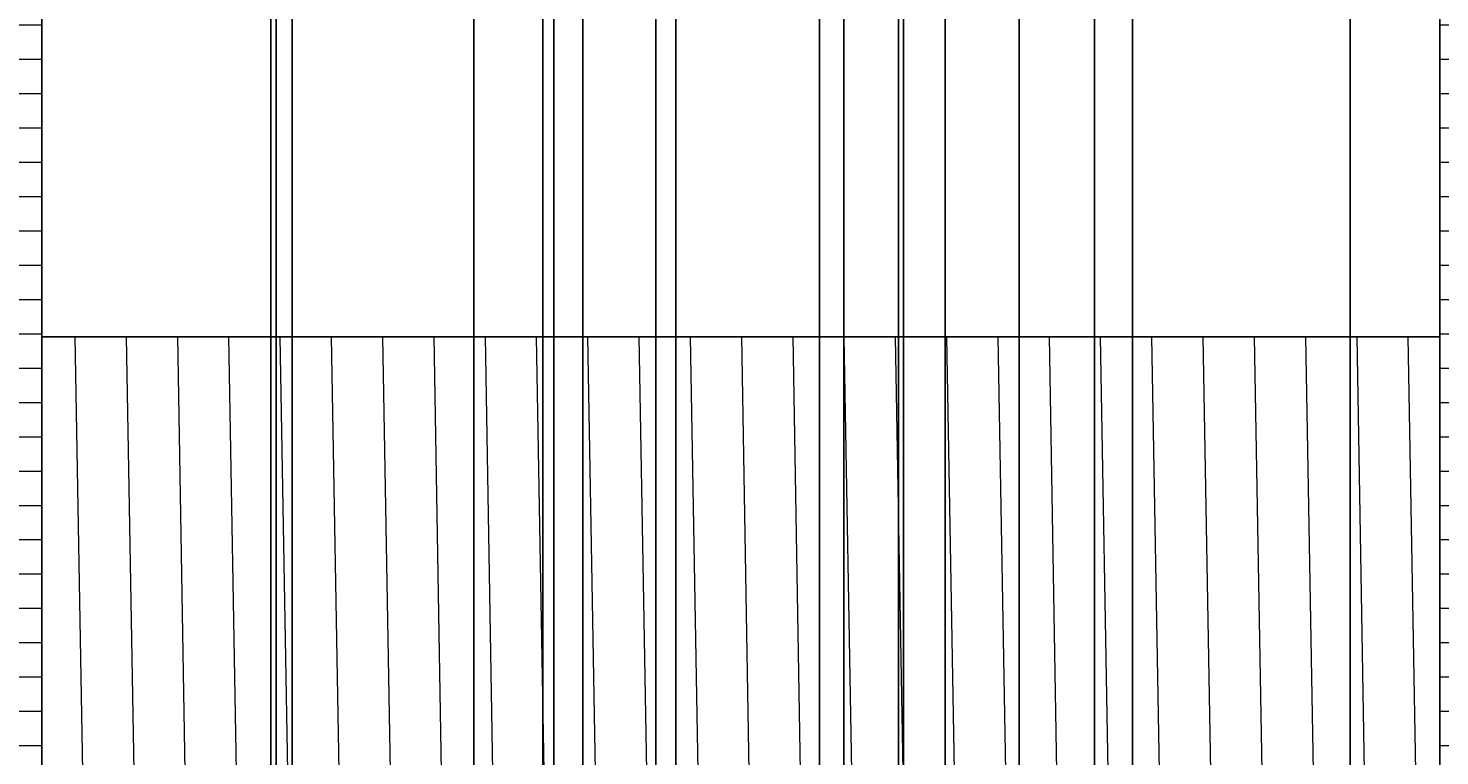
# Model space of a CAD drawing. Units: inches. Extents: x 241 to 943, y 109 to 1396.
# Tile 31 of 34: x 532 to 725, y 1180 to 1279. Entities that reach past the tile are written whole.
import ezdxf

# ---------------------------------------------------------------- set-up
doc = ezdxf.new("R2010")
doc.units = ezdxf.units.IN
doc.header["$MEASUREMENT"] = 0
for name, color, linetype, lineweight in [('A-ANNO-DIMS', 2, 'Continuous', 18), ('A-ELEV', 7, 'Continuous', 25), ('A-GLAZ', 4, 'Continuous', 18), ('A-WALL-PATT', 8, 'Continuous', 13)]:
    doc.layers.add(name, color=color, linetype=linetype, lineweight=lineweight)
doc.styles.get("Standard").update_dxf_attribs({"font": 'arial.ttf'})
doc.dimstyles.get("Standard").update_dxf_attribs({"dimtxt": 1.4375, "dimasz": 0.18, "dimexe": 0.18, "dimexo": 0.0625, "dimgap": 0.09, "dimtad": 0, "dimtih": 1, "dimtoh": 1, "dimdec": 4, "dimzin": 0, "dimdsep": 46, "dimlunit": 4, "dimtxsty": 'Standard', "dimcen": 0.09, "dimadec": 0, "dimazin": 0, "dimtfac": 1, "dimtdec": 4, "dimtofl": 0, "dimtmove": 0, "dimatfit": 3, "dimfxl": 1, "dimtolj": 1, "dimtzin": 0, "dimarcsym": 0})

# ---------------------------------------------------------------- blocks, each defined once
blk = doc.blocks.new('*D12')
at = {"layer": 'A-ANNO-DIMS', "color": 0, "lineweight": -2, "transparency": 16777216}
for p, q in [((530.23, 384.24), (530.23, 1395.05)), ((530.41, 1394.87), (587.56, 1394.87)), ((650.73, 1394.87), (593.58, 1394.87)), ((650.91, 384.24), (650.91, 1395.05))]:
    blk.add_line(p, q, dxfattribs=at)
at = {"layer": 'A-ANNO-DIMS', "color": 0, "transparency": 16777216}
for points in [[(530.41, 1394.9), (530.41, 1394.84), (530.23, 1394.87)], [(650.73, 1394.9), (650.73, 1394.84), (650.91, 1394.87)]]:
    blk.add_solid(points, dxfattribs=at)
at = {"layer": 'Defpoints', "color": 0, "transparency": 16777216}
for p in [(650.91, 1394.87), (530.23, 384.18), (650.91, 384.18)]:
    blk.add_point(p, dxfattribs=at)
at = {"layer": 'A-ANNO-DIMS', "color": 0, "transparency": 16777216, "insert": (590.57, 1394.87), "char_height": 1.438, "attachment_point": 5}
blk.add_mtext('\\A1;120.68', dxfattribs=at)
blk = doc.blocks.new('*D13')
at = {"layer": 'A-ANNO-DIMS', "color": 0, "lineweight": -2, "transparency": 16777216}
for p, q in [((650.91, 384.24), (650.91, 1395.05)), ((651.09, 1394.87), (656.14, 1394.87)), ((667.21, 1394.87), (662.16, 1394.87)), ((667.39, 290.06), (667.39, 1395.05))]:
    blk.add_line(p, q, dxfattribs=at)
at = {"layer": 'A-ANNO-DIMS', "color": 0, "transparency": 16777216}
for points in [[(651.09, 1394.9), (651.09, 1394.84), (650.91, 1394.87)], [(667.21, 1394.9), (667.21, 1394.84), (667.39, 1394.87)]]:
    blk.add_solid(points, dxfattribs=at)
at = {"layer": 'Defpoints', "color": 0, "transparency": 16777216}
for p in [(667.39, 1394.87), (650.91, 384.18), (667.39, 290)]:
    blk.add_point(p, dxfattribs=at)
at = {"layer": 'A-ANNO-DIMS', "color": 0, "transparency": 16777216, "insert": (659.15, 1394.87), "char_height": 1.438, "attachment_point": 5}
blk.add_mtext('\\A1;16.486', dxfattribs=at)
blk = doc.blocks.new('*D14')
at = {"layer": 'A-ANNO-DIMS', "color": 0, "lineweight": -2, "transparency": 16777216}
for p, q in [((667.39, 290.06), (667.39, 1395.05)), ((667.57, 1394.87), (727.7, 1394.87)), ((793.85, 1394.87), (733.72, 1394.87)), ((794.03, 290.06), (794.03, 1395.05))]:
    blk.add_line(p, q, dxfattribs=at)
at = {"layer": 'A-ANNO-DIMS', "color": 0, "transparency": 16777216}
for points in [[(667.57, 1394.9), (667.57, 1394.84), (667.39, 1394.87)], [(793.85, 1394.9), (793.85, 1394.84), (794.03, 1394.87)]]:
    blk.add_solid(points, dxfattribs=at)
at = {"layer": 'Defpoints', "color": 0, "transparency": 16777216}
for p in [(794.03, 1394.87), (667.39, 290), (794.03, 290)]:
    blk.add_point(p, dxfattribs=at)
at = {"layer": 'A-ANNO-DIMS', "color": 0, "transparency": 16777216, "insert": (730.71, 1394.87), "char_height": 1.438, "attachment_point": 5}
blk.add_mtext('\\A1;126.63', dxfattribs=at)
blk = doc.blocks.new('*D57')
at = {"layer": 'A-ANNO-DIMS', "color": 0, "lineweight": -2, "transparency": 16777216}
for p, q in [((508.31, 1070.92), (508.31, 1395.05)), ((508.49, 1394.87), (518.04, 1394.87)), ((533.77, 1394.87), (524.21, 1394.87)), ((533.95, 1108.23), (533.95, 1395.05))]:
    blk.add_line(p, q, dxfattribs=at)
at = {"layer": 'A-ANNO-DIMS', "color": 0, "transparency": 16777216}
for points in [[(508.49, 1394.9), (508.49, 1394.84), (508.31, 1394.87)], [(533.77, 1394.9), (533.77, 1394.84), (533.95, 1394.87)]]:
    blk.add_solid(points, dxfattribs=at)
at = {"layer": 'Defpoints', "color": 0, "transparency": 16777216}
for p in [(533.95, 1394.87), (533.95, 1108.17), (508.31, 1070.85)]:
    blk.add_point(p, dxfattribs=at)
at = {"layer": 'A-ANNO-DIMS', "color": 0, "transparency": 16777216, "insert": (521.13, 1394.87), "char_height": 1.438, "attachment_point": 5}
blk.add_mtext('\\A1;25.646', dxfattribs=at)
blk = doc.blocks.new('*D62')
at = {"layer": 'A-ANNO-DIMS', "color": 0, "lineweight": -2, "transparency": 16777216}
for p, q in [((424.11, 568.89), (424.11, 1395.05)), ((424.29, 1394.87), (492.35, 1394.87)), ((565.02, 1394.87), (496.96, 1394.87)), ((565.2, 568.89), (565.2, 1395.05))]:
    blk.add_line(p, q, dxfattribs=at)
at = {"layer": 'A-ANNO-DIMS', "color": 0, "transparency": 16777216}
for points in [[(424.29, 1394.9), (424.29, 1394.84), (424.11, 1394.87)], [(565.02, 1394.9), (565.02, 1394.84), (565.2, 1394.87)]]:
    blk.add_solid(points, dxfattribs=at)
at = {"layer": 'Defpoints', "color": 0, "transparency": 16777216}
for p in [(565.2, 1394.87), (424.11, 568.83), (565.2, 568.83)]:
    blk.add_point(p, dxfattribs=at)
at = {"layer": 'A-ANNO-DIMS', "color": 0, "transparency": 16777216, "insert": (494.66, 1394.87), "char_height": 1.438, "attachment_point": 5}
blk.add_mtext('\\A1;141.1', dxfattribs=at)
blk = doc.blocks.new('*D63')
at = {"layer": 'A-ANNO-DIMS', "color": 0, "lineweight": -2, "transparency": 16777216}
for p, q in [((651.6, 568.89), (651.6, 1395.05)), ((651.78, 1394.87), (719.84, 1394.87)), ((792.51, 1394.87), (724.45, 1394.87)), ((792.69, 568.89), (792.69, 1395.05))]:
    blk.add_line(p, q, dxfattribs=at)
at = {"layer": 'A-ANNO-DIMS', "color": 0, "transparency": 16777216}
for points in [[(651.78, 1394.9), (651.78, 1394.84), (651.6, 1394.87)], [(792.51, 1394.9), (792.51, 1394.84), (792.69, 1394.87)]]:
    blk.add_solid(points, dxfattribs=at)
at = {"layer": 'Defpoints', "color": 0, "transparency": 16777216}
for p in [(792.69, 1394.87), (651.6, 568.83), (792.69, 568.83)]:
    blk.add_point(p, dxfattribs=at)
at = {"layer": 'A-ANNO-DIMS', "color": 0, "transparency": 16777216, "insert": (722.14, 1394.87), "char_height": 1.438, "attachment_point": 5}
blk.add_mtext('\\A1;141.1', dxfattribs=at)
blk = doc.blocks.new('*D65')
at = {"layer": 'A-ANNO-DIMS', "color": 0, "lineweight": -2, "transparency": 16777216}
for p, q in [((424.11, 700.85), (424.11, 1395.05)), ((424.29, 1394.87), (505.52, 1394.87)), ((592.77, 1394.87), (511.54, 1394.87)), ((592.95, 700.85), (592.95, 1395.05))]:
    blk.add_line(p, q, dxfattribs=at)
at = {"layer": 'A-ANNO-DIMS', "color": 0, "transparency": 16777216}
for points in [[(424.29, 1394.9), (424.29, 1394.84), (424.11, 1394.87)], [(592.77, 1394.9), (592.77, 1394.84), (592.95, 1394.87)]]:
    blk.add_solid(points, dxfattribs=at)
at = {"layer": 'Defpoints', "color": 0, "transparency": 16777216}
for p in [(592.95, 1394.87), (424.11, 700.79), (592.95, 700.79)]:
    blk.add_point(p, dxfattribs=at)
at = {"layer": 'A-ANNO-DIMS', "color": 0, "transparency": 16777216, "insert": (508.53, 1394.87), "char_height": 1.438, "attachment_point": 5}
blk.add_mtext('\\A1;168.85', dxfattribs=at)
blk = doc.blocks.new('*D66')
at = {"layer": 'A-ANNO-DIMS', "color": 0, "lineweight": -2, "transparency": 16777216}
for p, q in [((617.76, 702.85), (617.76, 1395.05)), ((617.94, 1394.87), (680.69, 1394.87)), ((749.45, 1394.87), (686.7, 1394.87)), ((749.63, 702.85), (749.63, 1395.05))]:
    blk.add_line(p, q, dxfattribs=at)
at = {"layer": 'A-ANNO-DIMS', "color": 0, "transparency": 16777216}
for points in [[(617.94, 1394.9), (617.94, 1394.84), (617.76, 1394.87)], [(749.45, 1394.9), (749.45, 1394.84), (749.63, 1394.87)]]:
    blk.add_solid(points, dxfattribs=at)
at = {"layer": 'Defpoints', "color": 0, "transparency": 16777216}
for p in [(749.63, 1394.87), (617.76, 702.79), (749.63, 702.79)]:
    blk.add_point(p, dxfattribs=at)
at = {"layer": 'A-ANNO-DIMS', "color": 0, "transparency": 16777216, "insert": (683.7, 1394.87), "char_height": 1.438, "attachment_point": 5}
blk.add_mtext('\\A1;131.87', dxfattribs=at)
blk = doc.blocks.new('*D67')
at = {"layer": 'A-ANNO-DIMS', "color": 0, "lineweight": -2, "transparency": 16777216}
for p, q in [((389.04, 773.55), (389.04, 1395.05)), ((389.22, 1394.87), (495.34, 1394.87)), ((607.64, 1394.87), (501.52, 1394.87)), ((607.82, 773.55), (607.82, 1395.05))]:
    blk.add_line(p, q, dxfattribs=at)
at = {"layer": 'A-ANNO-DIMS', "color": 0, "transparency": 16777216}
for points in [[(389.22, 1394.9), (389.22, 1394.84), (389.04, 1394.87)], [(607.64, 1394.9), (607.64, 1394.84), (607.82, 1394.87)]]:
    blk.add_solid(points, dxfattribs=at)
at = {"layer": 'Defpoints', "color": 0, "transparency": 16777216}
for p in [(607.82, 1394.87), (389.04, 773.49), (607.82, 773.49)]:
    blk.add_point(p, dxfattribs=at)
at = {"layer": 'A-ANNO-DIMS', "color": 0, "transparency": 16777216, "insert": (498.43, 1394.87), "char_height": 1.438, "attachment_point": 5}
blk.add_mtext('\\A1;218.77', dxfattribs=at)
blk = doc.blocks.new('*D68')
at = {"layer": 'A-ANNO-DIMS', "color": 0, "lineweight": -2, "transparency": 16777216}
for p, q in [((617.76, 841.6), (617.76, 1395.05)), ((617.94, 1394.87), (702.22, 1394.87)), ((792.51, 1394.87), (708.23, 1394.87)), ((792.69, 841.6), (792.69, 1395.05))]:
    blk.add_line(p, q, dxfattribs=at)
at = {"layer": 'A-ANNO-DIMS', "color": 0, "transparency": 16777216}
for points in [[(617.94, 1394.9), (617.94, 1394.84), (617.76, 1394.87)], [(792.51, 1394.9), (792.51, 1394.84), (792.69, 1394.87)]]:
    blk.add_solid(points, dxfattribs=at)
at = {"layer": 'Defpoints', "color": 0, "transparency": 16777216}
for p in [(792.69, 1394.87), (617.76, 841.54), (792.69, 841.54)]:
    blk.add_point(p, dxfattribs=at)
at = {"layer": 'A-ANNO-DIMS', "color": 0, "transparency": 16777216, "insert": (705.23, 1394.87), "char_height": 1.438, "attachment_point": 5}
blk.add_mtext('\\A1;174.93', dxfattribs=at)
blk = doc.blocks.new('*D69')
at = {"layer": 'A-ANNO-DIMS', "color": 0, "lineweight": -2, "transparency": 16777216}
for p, q in [((389.04, 941.55), (389.04, 1395.05)), ((389.22, 1394.87), (476.28, 1394.87)), ((567.95, 1394.87), (480.9, 1394.87)), ((568.13, 941.55), (568.13, 1395.05))]:
    blk.add_line(p, q, dxfattribs=at)
at = {"layer": 'A-ANNO-DIMS', "color": 0, "transparency": 16777216}
for points in [[(389.22, 1394.9), (389.22, 1394.84), (389.04, 1394.87)], [(567.95, 1394.9), (567.95, 1394.84), (568.13, 1394.87)]]:
    blk.add_solid(points, dxfattribs=at)
at = {"layer": 'Defpoints', "color": 0, "transparency": 16777216}
for p in [(568.13, 1394.87), (389.04, 941.49), (568.13, 941.49)]:
    blk.add_point(p, dxfattribs=at)
at = {"layer": 'A-ANNO-DIMS', "color": 0, "transparency": 16777216, "insert": (478.59, 1394.87), "char_height": 1.438, "attachment_point": 5}
blk.add_mtext('\\A1;179.1', dxfattribs=at)
blk = doc.blocks.new('*D70')
at = {"layer": 'A-ANNO-DIMS', "color": 0, "lineweight": -2, "transparency": 16777216}
for p, q in [((603.87, 1009.6), (603.87, 1395.05)), ((604.05, 1394.87), (674.69, 1394.87)), ((751.33, 1394.87), (680.69, 1394.87)), ((751.51, 1009.6), (751.51, 1395.05))]:
    blk.add_line(p, q, dxfattribs=at)
at = {"layer": 'A-ANNO-DIMS', "color": 0, "transparency": 16777216}
for points in [[(604.05, 1394.9), (604.05, 1394.84), (603.87, 1394.87)], [(751.33, 1394.9), (751.33, 1394.84), (751.51, 1394.87)]]:
    blk.add_solid(points, dxfattribs=at)
at = {"layer": 'Defpoints', "color": 0, "transparency": 16777216}
for p in [(751.51, 1394.87), (603.87, 1009.54), (751.51, 1009.54)]:
    blk.add_point(p, dxfattribs=at)
at = {"layer": 'A-ANNO-DIMS', "color": 0, "transparency": 16777216, "insert": (677.69, 1394.87), "char_height": 1.438, "attachment_point": 5}
blk.add_mtext('\\A1;147.64', dxfattribs=at)
blk = doc.blocks.new('*D82')
at = {"layer": 'A-ANNO-DIMS', "color": 0, "lineweight": -2, "transparency": 16777216}
for p, q in [((565.2, 568.89), (565.2, 1395.05)), ((565.38, 1394.87), (605.89, 1394.87)), ((651.42, 1394.87), (610.91, 1394.87)), ((651.6, 568.89), (651.6, 1395.05))]:
    blk.add_line(p, q, dxfattribs=at)
at = {"layer": 'A-ANNO-DIMS', "color": 0, "transparency": 16777216}
for points in [[(565.38, 1394.9), (565.38, 1394.84), (565.2, 1394.87)], [(651.42, 1394.9), (651.42, 1394.84), (651.6, 1394.87)]]:
    blk.add_solid(points, dxfattribs=at)
at = {"layer": 'Defpoints', "color": 0, "transparency": 16777216}
for p in [(651.6, 1394.87), (565.2, 568.83), (651.6, 568.83)]:
    blk.add_point(p, dxfattribs=at)
at = {"layer": 'A-ANNO-DIMS', "color": 0, "transparency": 16777216, "insert": (608.4, 1394.87), "char_height": 1.438, "attachment_point": 5}
blk.add_mtext('\\A1;86.40', dxfattribs=at)
blk = doc.blocks.new('*D83')
at = {"layer": 'A-ANNO-DIMS', "color": 0, "lineweight": -2, "transparency": 16777216}
for p, q in [((592.95, 700.85), (592.95, 1395.05)), ((593.13, 1394.87), (602.27, 1394.87)), ((617.58, 1394.87), (608.45, 1394.87)), ((617.76, 702.85), (617.76, 1395.05))]:
    blk.add_line(p, q, dxfattribs=at)
at = {"layer": 'A-ANNO-DIMS', "color": 0, "transparency": 16777216}
for points in [[(593.13, 1394.9), (593.13, 1394.84), (592.95, 1394.87)], [(617.58, 1394.9), (617.58, 1394.84), (617.76, 1394.87)]]:
    blk.add_solid(points, dxfattribs=at)
at = {"layer": 'Defpoints', "color": 0, "transparency": 16777216}
for p in [(617.76, 1394.87), (617.76, 702.79), (592.95, 700.79)]:
    blk.add_point(p, dxfattribs=at)
at = {"layer": 'A-ANNO-DIMS', "color": 0, "transparency": 16777216, "insert": (605.36, 1394.87), "char_height": 1.438, "attachment_point": 5}
blk.add_mtext('\\A1;24.805', dxfattribs=at)
blk = doc.blocks.new('*D89')
at = {"layer": 'A-ANNO-DIMS', "color": 0, "lineweight": -2, "transparency": 16777216}
for p, q in [((377.04, 841.6), (377.04, 1395.05)), ((377.22, 1394.87), (494.32, 1394.87)), ((617.58, 1394.87), (500.48, 1394.87)), ((617.76, 841.6), (617.76, 1395.05))]:
    blk.add_line(p, q, dxfattribs=at)
at = {"layer": 'A-ANNO-DIMS', "color": 0, "transparency": 16777216}
for points in [[(377.22, 1394.9), (377.22, 1394.84), (377.04, 1394.87)], [(617.58, 1394.9), (617.58, 1394.84), (617.76, 1394.87)]]:
    blk.add_solid(points, dxfattribs=at)
at = {"layer": 'Defpoints', "color": 0, "transparency": 16777216}
for p in [(617.76, 1394.87), (377.04, 841.54), (617.76, 841.54)]:
    blk.add_point(p, dxfattribs=at)
at = {"layer": 'A-ANNO-DIMS', "color": 0, "transparency": 16777216, "insert": (497.4, 1394.87), "char_height": 1.438, "attachment_point": 5}
blk.add_mtext('\\A1;240.72', dxfattribs=at)
blk = doc.blocks.new('*D90')
at = {"layer": 'A-ANNO-DIMS', "color": 0, "lineweight": -2, "transparency": 16777216}
for p, q in [((568.13, 941.55), (568.13, 1395.05)), ((568.31, 1394.87), (582.92, 1394.87)), ((603.69, 1394.87), (589.08, 1394.87)), ((603.87, 902.92), (603.87, 1395.05))]:
    blk.add_line(p, q, dxfattribs=at)
at = {"layer": 'A-ANNO-DIMS', "color": 0, "transparency": 16777216}
for points in [[(568.31, 1394.9), (568.31, 1394.84), (568.13, 1394.87)], [(603.69, 1394.9), (603.69, 1394.84), (603.87, 1394.87)]]:
    blk.add_solid(points, dxfattribs=at)
at = {"layer": 'Defpoints', "color": 0, "transparency": 16777216}
for p in [(603.87, 1394.87), (568.13, 941.49), (603.87, 902.85)]:
    blk.add_point(p, dxfattribs=at)
at = {"layer": 'A-ANNO-DIMS', "color": 0, "transparency": 16777216, "insert": (586, 1394.87), "char_height": 1.438, "attachment_point": 5}
blk.add_mtext('\\A1;35.735', dxfattribs=at)
blk = doc.blocks.new('*D99')
at = {"layer": 'A-ANNO-DIMS', "color": 0, "lineweight": -2, "transparency": 16777216}
for p, q in [((417.09, 181.71), (417.09, 1395.05)), ((417.27, 1394.87), (539.16, 1394.87)), ((667.21, 1394.87), (545.33, 1394.87)), ((667.39, 214.58), (667.39, 1395.05))]:
    blk.add_line(p, q, dxfattribs=at)
at = {"layer": 'A-ANNO-DIMS', "color": 0, "transparency": 16777216}
for points in [[(417.27, 1394.9), (417.27, 1394.84), (417.09, 1394.87)], [(667.21, 1394.9), (667.21, 1394.84), (667.39, 1394.87)]]:
    blk.add_solid(points, dxfattribs=at)
at = {"layer": 'Defpoints', "color": 0, "transparency": 16777216}
for p in [(667.39, 1394.87), (667.39, 214.52), (417.09, 181.65)]:
    blk.add_point(p, dxfattribs=at)
at = {"layer": 'A-ANNO-DIMS', "color": 0, "transparency": 16777216, "insert": (542.24, 1394.87), "char_height": 1.438, "attachment_point": 5}
blk.add_mtext('\\A1;250.30', dxfattribs=at)
blk = doc.blocks.new('*D104')
at = {"layer": 'A-ANNO-DIMS', "color": 0, "lineweight": -2, "transparency": 16777216}
for p, q in [((533.95, 1108.23), (533.95, 1395.05)), ((534.13, 1394.87), (546.87, 1394.87)), ((565.77, 1394.87), (553.03, 1394.87)), ((565.95, 1110.23), (565.95, 1395.05))]:
    blk.add_line(p, q, dxfattribs=at)
at = {"layer": 'A-ANNO-DIMS', "color": 0, "transparency": 16777216}
for points in [[(534.13, 1394.9), (534.13, 1394.84), (533.95, 1394.87)], [(565.77, 1394.9), (565.77, 1394.84), (565.95, 1394.87)]]:
    blk.add_solid(points, dxfattribs=at)
at = {"layer": 'Defpoints', "color": 0, "transparency": 16777216}
for p in [(565.95, 1394.87), (565.95, 1110.17), (533.95, 1108.17)]:
    blk.add_point(p, dxfattribs=at)
at = {"layer": 'A-ANNO-DIMS', "color": 0, "transparency": 16777216, "insert": (549.95, 1394.87), "char_height": 1.438, "attachment_point": 5}
blk.add_mtext('\\A1;31.995', dxfattribs=at)
blk = doc.blocks.new('*D105')
at = {"layer": 'A-ANNO-DIMS', "color": 0, "lineweight": -2, "transparency": 16777216}
for p, q in [((565.95, 1110.23), (565.95, 1395.05)), ((566.13, 1394.87), (581.08, 1394.87)), ((602.18, 1394.87), (587.23, 1394.87)), ((602.36, 1110.23), (602.36, 1395.05))]:
    blk.add_line(p, q, dxfattribs=at)
at = {"layer": 'A-ANNO-DIMS', "color": 0, "transparency": 16777216}
for points in [[(566.13, 1394.9), (566.13, 1394.84), (565.95, 1394.87)], [(602.18, 1394.9), (602.18, 1394.84), (602.36, 1394.87)]]:
    blk.add_solid(points, dxfattribs=at)
at = {"layer": 'Defpoints', "color": 0, "transparency": 16777216}
for p in [(602.36, 1394.87), (565.95, 1110.17), (602.36, 1110.17)]:
    blk.add_point(p, dxfattribs=at)
at = {"layer": 'A-ANNO-DIMS', "color": 0, "transparency": 16777216, "insert": (584.15, 1394.87), "char_height": 1.438, "attachment_point": 5}
blk.add_mtext('\\A1;36.415', dxfattribs=at)
blk = doc.blocks.new('*D106')
at = {"layer": 'A-ANNO-DIMS', "color": 0, "lineweight": -2, "transparency": 16777216}
for p, q in [((602.36, 1110.23), (602.36, 1395.05)), ((602.54, 1394.87), (608.99, 1394.87)), ((620.34, 1394.87), (613.89, 1394.87)), ((620.52, 1110.23), (620.52, 1395.05))]:
    blk.add_line(p, q, dxfattribs=at)
at = {"layer": 'A-ANNO-DIMS', "color": 0, "transparency": 16777216}
for points in [[(602.54, 1394.9), (602.54, 1394.84), (602.36, 1394.87)], [(620.34, 1394.9), (620.34, 1394.84), (620.52, 1394.87)]]:
    blk.add_solid(points, dxfattribs=at)
at = {"layer": 'Defpoints', "color": 0, "transparency": 16777216}
for p in [(620.52, 1394.87), (602.36, 1110.17), (620.52, 1110.17)]:
    blk.add_point(p, dxfattribs=at)
at = {"layer": 'A-ANNO-DIMS', "color": 0, "transparency": 16777216, "insert": (611.44, 1394.87), "char_height": 1.438, "attachment_point": 5}
blk.add_mtext('\\A1;18.16', dxfattribs=at)
blk = doc.blocks.new('*D107')
at = {"layer": 'A-ANNO-DIMS', "color": 0, "lineweight": -2, "transparency": 16777216}
for p, q in [((620.52, 1110.23), (620.52, 1395.05)), ((620.7, 1394.87), (628.91, 1394.87)), ((643.27, 1394.87), (635.07, 1394.87)), ((643.45, 1110.23), (643.45, 1395.05))]:
    blk.add_line(p, q, dxfattribs=at)
at = {"layer": 'A-ANNO-DIMS', "color": 0, "transparency": 16777216}
for points in [[(620.7, 1394.9), (620.7, 1394.84), (620.52, 1394.87)], [(643.27, 1394.9), (643.27, 1394.84), (643.45, 1394.87)]]:
    blk.add_solid(points, dxfattribs=at)
at = {"layer": 'Defpoints', "color": 0, "transparency": 16777216}
for p in [(643.45, 1394.87), (620.52, 1110.17), (643.45, 1110.17)]:
    blk.add_point(p, dxfattribs=at)
at = {"layer": 'A-ANNO-DIMS', "color": 0, "transparency": 16777216, "insert": (631.99, 1394.87), "char_height": 1.438, "attachment_point": 5}
blk.add_mtext('\\A1;22.932', dxfattribs=at)
blk = doc.blocks.new('*D108')
at = {"layer": 'A-ANNO-DIMS', "color": 0, "lineweight": -2, "transparency": 16777216}
for p, q in [((643.45, 1110.23), (643.45, 1395.05)), ((643.63, 1394.87), (660.66, 1394.87)), ((682.69, 1394.87), (665.67, 1394.87)), ((682.87, 1110.23), (682.87, 1395.05))]:
    blk.add_line(p, q, dxfattribs=at)
at = {"layer": 'A-ANNO-DIMS', "color": 0, "transparency": 16777216}
for points in [[(643.63, 1394.9), (643.63, 1394.84), (643.45, 1394.87)], [(682.69, 1394.9), (682.69, 1394.84), (682.87, 1394.87)]]:
    blk.add_solid(points, dxfattribs=at)
at = {"layer": 'Defpoints', "color": 0, "transparency": 16777216}
for p in [(682.87, 1394.87), (643.45, 1110.17), (682.87, 1110.17)]:
    blk.add_point(p, dxfattribs=at)
at = {"layer": 'A-ANNO-DIMS', "color": 0, "transparency": 16777216, "insert": (663.16, 1394.87), "char_height": 1.438, "attachment_point": 5}
blk.add_mtext('\\A1;39.42', dxfattribs=at)
blk = doc.blocks.new('*D109')
at = {"layer": 'A-ANNO-DIMS', "color": 0, "lineweight": -2, "transparency": 16777216}
for p, q in [((682.87, 1110.23), (682.87, 1395.05)), ((683.05, 1394.87), (701.31, 1394.87)), ((724.64, 1394.87), (706.39, 1394.87)), ((724.82, 1108.23), (724.82, 1395.05))]:
    blk.add_line(p, q, dxfattribs=at)
at = {"layer": 'A-ANNO-DIMS', "color": 0, "transparency": 16777216}
for points in [[(683.05, 1394.9), (683.05, 1394.84), (682.87, 1394.87)], [(724.64, 1394.9), (724.64, 1394.84), (724.82, 1394.87)]]:
    blk.add_solid(points, dxfattribs=at)
at = {"layer": 'Defpoints', "color": 0, "transparency": 16777216}
for p in [(724.82, 1394.87), (682.87, 1110.17), (724.82, 1108.17)]:
    blk.add_point(p, dxfattribs=at)
at = {"layer": 'A-ANNO-DIMS', "color": 0, "transparency": 16777216, "insert": (703.85, 1394.87), "char_height": 1.438, "attachment_point": 5}
blk.add_mtext('\\A1;41.94', dxfattribs=at)
blk = doc.blocks.new('*D113')
at = {"layer": 'A-ANNO-DIMS', "color": 0, "lineweight": -2, "transparency": 16777216}
for p, q in [((603.87, 902.92), (603.87, 1395.05)), ((604.05, 1394.87), (618.91, 1394.87)), ((639.93, 1394.87), (625.07, 1394.87)), ((640.11, 902.92), (640.11, 1395.05))]:
    blk.add_line(p, q, dxfattribs=at)
at = {"layer": 'A-ANNO-DIMS', "color": 0, "transparency": 16777216}
for points in [[(604.05, 1394.9), (604.05, 1394.84), (603.87, 1394.87)], [(639.93, 1394.9), (639.93, 1394.84), (640.11, 1394.87)]]:
    blk.add_solid(points, dxfattribs=at)
at = {"layer": 'Defpoints', "color": 0, "transparency": 16777216}
for p in [(640.11, 1394.87), (603.87, 902.85), (640.11, 902.85)]:
    blk.add_point(p, dxfattribs=at)
at = {"layer": 'A-ANNO-DIMS', "color": 0, "transparency": 16777216, "insert": (621.99, 1394.87), "char_height": 1.438, "attachment_point": 5}
blk.add_mtext('\\A1;36.245', dxfattribs=at)
blk = doc.blocks.new('*D114')
at = {"layer": 'A-ANNO-DIMS', "color": 0, "lineweight": -2, "transparency": 16777216}
for p, q in [((640.11, 902.92), (640.11, 1395.05)), ((640.29, 1394.87), (646.25, 1394.87)), ((657.11, 1394.87), (651.15, 1394.87)), ((657.29, 902.92), (657.29, 1395.05))]:
    blk.add_line(p, q, dxfattribs=at)
at = {"layer": 'A-ANNO-DIMS', "color": 0, "transparency": 16777216}
for points in [[(640.29, 1394.9), (640.29, 1394.84), (640.11, 1394.87)], [(657.11, 1394.9), (657.11, 1394.84), (657.29, 1394.87)]]:
    blk.add_solid(points, dxfattribs=at)
at = {"layer": 'Defpoints', "color": 0, "transparency": 16777216}
for p in [(657.29, 1394.87), (640.11, 902.85), (657.29, 902.85)]:
    blk.add_point(p, dxfattribs=at)
at = {"layer": 'A-ANNO-DIMS', "color": 0, "transparency": 16777216, "insert": (648.7, 1394.87), "char_height": 1.438, "attachment_point": 5}
blk.add_mtext('\\A1;17.18', dxfattribs=at)
blk = doc.blocks.new('*D115')
at = {"layer": 'A-ANNO-DIMS', "color": 0, "lineweight": -2, "transparency": 16777216}
for p, q in [((657.29, 902.92), (657.29, 1395.05)), ((657.47, 1394.87), (664.4, 1394.87)), ((677.51, 1394.87), (670.58, 1394.87)), ((677.69, 902.92), (677.69, 1395.05))]:
    blk.add_line(p, q, dxfattribs=at)
at = {"layer": 'A-ANNO-DIMS', "color": 0, "transparency": 16777216}
for points in [[(657.47, 1394.9), (657.47, 1394.84), (657.29, 1394.87)], [(677.51, 1394.9), (677.51, 1394.84), (677.69, 1394.87)]]:
    blk.add_solid(points, dxfattribs=at)
at = {"layer": 'Defpoints', "color": 0, "transparency": 16777216}
for p in [(677.69, 1394.87), (657.29, 902.85), (677.69, 902.85)]:
    blk.add_point(p, dxfattribs=at)
at = {"layer": 'A-ANNO-DIMS', "color": 0, "transparency": 16777216, "insert": (667.49, 1394.87), "char_height": 1.438, "attachment_point": 5}
blk.add_mtext('\\A1;20.396', dxfattribs=at)
blk = doc.blocks.new('*D116')
at = {"layer": 'A-ANNO-DIMS', "color": 0, "lineweight": -2, "transparency": 16777216}
for p, q in [((677.69, 902.92), (677.69, 1395.05)), ((677.87, 1394.87), (692.06, 1394.87)), ((712.4, 1394.87), (698.22, 1394.87)), ((712.58, 902.92), (712.58, 1395.05))]:
    blk.add_line(p, q, dxfattribs=at)
at = {"layer": 'A-ANNO-DIMS', "color": 0, "transparency": 16777216}
for points in [[(677.87, 1394.9), (677.87, 1394.84), (677.69, 1394.87)], [(712.4, 1394.9), (712.4, 1394.84), (712.58, 1394.87)]]:
    blk.add_solid(points, dxfattribs=at)
at = {"layer": 'Defpoints', "color": 0, "transparency": 16777216}
for p in [(712.58, 1394.87), (677.69, 902.85), (712.58, 902.85)]:
    blk.add_point(p, dxfattribs=at)
at = {"layer": 'A-ANNO-DIMS', "color": 0, "transparency": 16777216, "insert": (695.14, 1394.87), "char_height": 1.438, "attachment_point": 5}
blk.add_mtext('\\A1;34.895', dxfattribs=at)
blk = doc.blocks.new('*D117')
at = {"layer": 'A-ANNO-DIMS', "color": 0, "lineweight": -2, "transparency": 16777216}
for p, q in [((712.58, 902.92), (712.58, 1395.05)), ((712.76, 1394.87), (729.54, 1394.87)), ((751.33, 1394.87), (734.55, 1394.87)), ((751.51, 902.92), (751.51, 1395.05))]:
    blk.add_line(p, q, dxfattribs=at)
at = {"layer": 'A-ANNO-DIMS', "color": 0, "transparency": 16777216}
for points in [[(712.76, 1394.9), (712.76, 1394.84), (712.58, 1394.87)], [(751.33, 1394.9), (751.33, 1394.84), (751.51, 1394.87)]]:
    blk.add_solid(points, dxfattribs=at)
at = {"layer": 'Defpoints', "color": 0, "transparency": 16777216}
for p in [(751.51, 1394.87), (712.58, 902.85), (751.51, 902.85)]:
    blk.add_point(p, dxfattribs=at)
at = {"layer": 'A-ANNO-DIMS', "color": 0, "transparency": 16777216, "insert": (732.05, 1394.87), "char_height": 1.438, "attachment_point": 5}
blk.add_mtext('\\A1;38.92', dxfattribs=at)

msp = doc.modelspace()

# ---------------------------------------------------------------- hatches: boundary and pattern name
at = {"layer": 'A-WALL-PATT'}
h = msp.add_hatch(dxfattribs=at)
h.set_pattern_fill('GRATE', color=256, scale=150)
h.paths.add_polyline_path([(747.7579, 1238.8538), (747.7579, 1275.9142), (747.7579, 1336.1154), (508.3064, 1336.1154), (508.3064, 1275.9142), (508.3064, 1238.8538), (508.3064, 1177.5382), (508.3064, 1109.4916), (508.3064, 1070.8538), (553.5166, 1070.8538), (749.6328, 1070.8538)])
h.paths.add_polyline_path([(533.952, 1108.1686), (533.952, 1177.7336), (533.952, 1303.0286), (724.819, 1303.0286), (724.819, 1108.1686)], flags=16)
h.paths.add_polyline_path([(535.952, 1110.1686), (535.952, 1175.7336), (722.819, 1175.7336), (722.819, 1110.1686)], flags=0)
h.paths.add_polyline_path([(643.4534, 1134.0739), (622.521, 1134.0739), (622.521, 1136.0739), (643.4534, 1136.0739)], flags=0)
h.paths.add_polyline_path([(617.7594, 568.8295), (617.7594, 734.8538), (377.0391, 734.8538), (377.0391, 566.8538), (377.0391, 400.8295), (417.0913, 400.8295), (618.9643, 400.8295)])
h.paths.add_polyline_path([(424.1086, 496.4395), (424.1086, 568.8295), (565.2023, 568.8295), (565.2023, 496.4395)], flags=16)
h.paths.add_polyline_path([(426.1086, 498.4395), (426.1086, 566.8295), (563.2023, 566.8295), (563.2023, 508.9074), (563.2023, 498.4395)], flags=0)
h.paths.add_polyline_path([(508.0803, 508.9074), (508.0803, 519.3754), (450.9259, 519.3754), (450.9259, 525.3816), (445.5808, 525.3816, -1), (445.5808, 527.3816), (450.9259, 527.3816), (450.9259, 566.8295), (508.0803, 566.8295), (537.4269, 566.8295), (537.4269, 508.9074)], flags=0)
h.paths.add_polyline_path([(506.0803, 521.3754), (452.9259, 521.3754), (452.9259, 564.8295), (506.0803, 564.8295)], flags=0)
h.paths.add_polyline_path([(424.1086, 628.4013), (424.1086, 700.7912), (592.9542, 700.7912), (592.9542, 628.4013)], flags=16)
h.paths.add_polyline_path([(426.1086, 630.4013), (426.1086, 698.7912), (590.8792, 698.7912), (590.8792, 630.4013)], flags=0)
h.paths.add_polyline_path([(508.1906, 651.3371), (508.0803, 651.3371), (450.9259, 651.3371), (428.0291, 651.3371), (428.0291, 698.7912), (451.9767, 698.7912), (508.0803, 698.7912), (537.4269, 698.7912), (563.2023, 698.7912), (563.2023, 659.3434), (563.9297, 659.3434), (563.9297, 651.3371)], flags=0)
h.paths.add_polyline_path([(506.0803, 653.3371), (452.9259, 653.3371), (452.9259, 657.3434), (445.5808, 657.3434, -1), (445.5808, 659.3434), (452.9259, 659.3434), (452.9259, 696.7912), (506.0803, 696.7912)], flags=0)
h = msp.add_hatch(dxfattribs=at)
h.set_pattern_fill('ANSI31', color=256, scale=56, angle=46)
h.paths.add_polyline_path([(508.3064, 1275.9142), (377.0391, 1275.9142), (377.0391, 1238.8538), (508.3064, 1238.8538)])
h.paths.add_polyline_path([(724.819, 1237.0695), (533.952, 1237.0695), (533.952, 1177.7336), (724.819, 1177.7336)])

# ---------------------------------------------------------------- linework, layer by layer
at = {"layer": 'A-ELEV'}
msp.add_line((533.952, 1237.0695), (724.819, 1237.0695), dxfattribs=at)
at = {"layer": 'A-GLAZ'}
msp.add_lwpolyline([(533.952, 1303.0286), (724.819, 1303.0286), (724.819, 1108.1686), (533.952, 1108.1686)], close=True, dxfattribs=at)

# ---------------------------------------------------------------- dimensions: what is measured, and where the dimension line sits
at = {"layer": 'A-ANNO-DIMS'}
for base, p1, p2, override, picture, middle in [((617.7594, 1394.8654), (377.0391, 841.5382), (617.7594, 841.5382), {"dimdec": 2, "dimlfac": 1, "dimrnd": 0, "dimzin": 0, "dimdsep": 46, "dimlunit": 2}, '*D89', (497.3993, 1394.8654)), ((607.8162, 1394.8654), (389.0429, 773.4916), (607.8162, 773.4916), {"dimdec": 2, "dimlfac": 1, "dimrnd": 0, "dimzin": 0, "dimdsep": 46, "dimlunit": 2}, '*D67', (498.4295, 1394.8654)), ((568.1348, 1394.8654), (389.0429, 941.4916), (568.1348, 941.4916), {"dimdec": 1, "dimlfac": 1, "dimrnd": 0, "dimzin": 0, "dimdsep": 46, "dimlunit": 2}, '*D69', (478.5888, 1394.8654)), ((667.3935, 1394.8654), (417.0913, 181.649), (667.3935, 214.5189), {"dimdec": 2, "dimlfac": 1, "dimrnd": 0, "dimzin": 0, "dimdsep": 46, "dimlunit": 2}, '*D99', (542.2424, 1394.8654)), ((565.2023, 1394.8654), (424.1086, 568.8295), (565.2023, 568.8295), {"dimdec": 1, "dimlfac": 1, "dimrnd": 0, "dimzin": 0, "dimdsep": 46, "dimlunit": 2}, '*D62', (494.6554, 1394.8654)), ((592.9542, 1394.8654), (424.1086, 700.7912), (592.9542, 700.7912), {"dimdec": 2, "dimlfac": 1, "dimrnd": 0, "dimzin": 0, "dimdsep": 46, "dimlunit": 2}, '*D65', (508.5314, 1394.8654)), ((533.952, 1394.8654), (508.3064, 1070.8538), (533.952, 1108.1686), {"dimdec": 3, "dimlfac": 1, "dimrnd": 0, "dimzin": 0, "dimdsep": 46, "dimlunit": 2}, '*D57', (521.1292, 1394.8654)), ((650.907, 1394.8654), (530.2303, 384.1784), (650.907, 384.1784), {"dimdec": 2, "dimlfac": 1, "dimrnd": 0, "dimzin": 0, "dimdsep": 46, "dimlunit": 2}, '*D12', (590.5686, 1394.8654)), ((565.947, 1394.8654), (533.952, 1108.1686), (565.947, 1110.1686), {"dimdec": 3, "dimlfac": 1, "dimrnd": 0, "dimzin": 0, "dimdsep": 46, "dimlunit": 2}, '*D104', (549.9495, 1394.8654)), ((651.5974, 1394.8654), (565.2023, 568.8295), (651.5974, 568.8295), {"dimdec": 2, "dimlfac": 1, "dimrnd": 0, "dimzin": 0, "dimdsep": 46, "dimlunit": 2}, '*D82', (608.3998, 1394.8654)), ((602.3616, 1394.8654), (565.947, 1110.1686), (602.3616, 1110.1686), {"dimdec": 3, "dimlfac": 1, "dimrnd": 0, "dimzin": 0, "dimdsep": 46, "dimlunit": 2}, '*D105', (584.1543, 1394.8654)), ((603.8694, 1394.8654), (568.1348, 941.4916), (603.8694, 902.8538), {"dimdec": 3, "dimlfac": 1, "dimrnd": 0, "dimzin": 0, "dimdsep": 46, "dimlunit": 2}, '*D90', (586.0021, 1394.8654)), ((617.7594, 1394.8654), (592.9542, 700.7912), (617.7594, 702.7912), {"dimdec": 3, "dimlfac": 1, "dimrnd": 0, "dimzin": 0, "dimdsep": 46, "dimlunit": 2}, '*D83', (605.3568, 1394.8654)), ((620.521, 1394.8654), (602.3616, 1110.1686), (620.521, 1110.1686), {"dimdec": 2, "dimlfac": 1, "dimrnd": 0, "dimzin": 0, "dimdsep": 46, "dimlunit": 2}, '*D106', (611.4413, 1394.8654)), ((751.5078, 1394.8654), (603.8694, 1009.5382), (751.5078, 1009.5382), {"dimdec": 2, "dimlfac": 1, "dimrnd": 0, "dimzin": 0, "dimdsep": 46, "dimlunit": 2}, '*D70', (677.6886, 1394.8654)), ((640.1141, 1394.8654), (603.8694, 902.8538), (640.1141, 902.8538), {"dimdec": 3, "dimlfac": 1, "dimrnd": 0, "dimzin": 0, "dimdsep": 46, "dimlunit": 2}, '*D113', (621.9918, 1394.8654)), ((749.6328, 1394.8654), (617.7594, 702.7912), (749.6328, 702.7912), {"dimdec": 2, "dimlfac": 1, "dimrnd": 0, "dimzin": 0, "dimdsep": 46, "dimlunit": 2}, '*D66', (683.6961, 1394.8654)), ((792.691, 1394.8654), (617.7594, 841.5382), (792.691, 841.5382), {"dimdec": 2, "dimlfac": 1, "dimrnd": 0, "dimzin": 0, "dimdsep": 46, "dimlunit": 2}, '*D68', (705.2252, 1394.8654)), ((643.4534, 1394.8654), (620.521, 1110.1686), (643.4534, 1110.1686), {"dimdec": 3, "dimlfac": 1, "dimrnd": 0, "dimzin": 0, "dimdsep": 46, "dimlunit": 2}, '*D107', (631.9872, 1394.8654)), ((657.2925, 1394.8654), (640.1141, 902.8538), (657.2925, 902.8538), {"dimdec": 2, "dimlfac": 1, "dimrnd": 0, "dimzin": 0, "dimdsep": 46, "dimlunit": 2}, '*D114', (648.7033, 1394.8654)), ((682.8748, 1394.8654), (643.4534, 1110.1686), (682.8748, 1110.1686), {"dimdec": 2, "dimlfac": 1, "dimrnd": 0, "dimzin": 0, "dimdsep": 46, "dimlunit": 2}, '*D108', (663.1641, 1394.8654)), ((667.39345, 1394.86544), (650.90697, 384.17836), (667.39345, 289.99842), {"dimdec": 3, "dimlfac": 1, "dimrnd": 0, "dimzin": 0, "dimdsep": 46, "dimlunit": 2}, '*D13', (659.15021, 1394.86544)), ((792.691, 1394.8654), (651.5974, 568.8295), (792.691, 568.8295), {"dimdec": 1, "dimlfac": 1, "dimrnd": 0, "dimzin": 0, "dimdsep": 46, "dimlunit": 2}, '*D63', (722.1442, 1394.8654)), ((677.6886, 1394.8654), (657.2925, 902.8538), (677.6886, 902.8538), {"dimdec": 3, "dimlfac": 1, "dimrnd": 0, "dimzin": 0, "dimdsep": 46, "dimlunit": 2}, '*D115', (667.4905, 1394.8654)), ((794.0275, 1394.8654), (667.3935, 289.9984), (794.0275, 289.9984), {"dimdec": 2, "dimlfac": 1, "dimrnd": 0, "dimzin": 0, "dimdsep": 46, "dimlunit": 2}, '*D14', (730.7105, 1394.8654)), ((712.5839, 1394.8654), (677.6886, 902.8538), (712.5839, 902.8538), {"dimdec": 3, "dimlfac": 1, "dimrnd": 0, "dimzin": 0, "dimdsep": 46, "dimlunit": 2}, '*D116', (695.1363, 1394.8654)), ((724.819, 1394.8654), (682.8748, 1110.1686), (724.819, 1108.1686), {"dimdec": 2, "dimlfac": 1, "dimrnd": 0, "dimzin": 0, "dimdsep": 46, "dimlunit": 2}, '*D109', (703.8469, 1394.8654)), ((751.5078, 1394.8654), (712.5839, 902.8538), (751.5078, 902.8538), {"dimdec": 2, "dimlfac": 1, "dimrnd": 0, "dimzin": 0, "dimdsep": 46, "dimlunit": 2}, '*D117', (732.0459, 1394.8654))]:
    dim = msp.add_linear_dim(base=base, p1=p1, p2=p2, dimstyle='Standard', override=override, dxfattribs=at)
    dim.commit()
    dim.dimension.update_dxf_attribs({"geometry": picture, "text_midpoint": middle})

doc.saveas('drawing.dxf')
